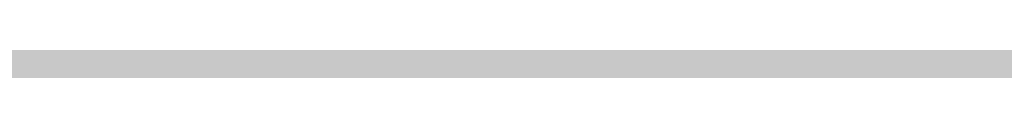
# Model space of a CAD drawing. Units: millimetres. Extents: x 0 to 2267, y 0 to 1823.
# Tile 242 of 256: x 1842.748 to 1843.095, y 1127.4185 to 1127.4234. Entities that reach past the tile are written whole.
import ezdxf

# ---------------------------------------------------------------- set-up
doc = ezdxf.new("R2010")
doc.units = ezdxf.units.MM
doc.header["$MEASUREMENT"] = 0
doc.layers.add('M-HATC', color=252, linetype='Continuous', lineweight=18)

msp = doc.modelspace()

# ---------------------------------------------------------------- hatches: boundary and pattern name
at = {"layer": 'M-HATC'}
h = msp.add_hatch(color=256, dxfattribs=at)
h.dxf.hatch_style = 1
h.paths.add_polyline_path([(2055.77105, 1603.06204), (1381.08677, 1603.06204), (1381.08677, 1598.06204), (2055.77105, 1598.06204)])
h.paths.add_polyline_path([(2055.77105, 1598.06204), (1381.08677, 1598.06204), (1381.08677, 1593.06204), (2055.77105, 1593.06204)])
h.paths.add_polyline_path([(2051.30737, 1536.76088), (1385.55044, 1536.76088), (1385.55044, 1526.76088), (1387.55044, 1526.76088), (1388.53662, 1525.05276), (1385.33187, 1521.23348), (1385.33187, 1521.22256), (2050.25417, 1522.74913), (2048.32119, 1525.05276), (2049.30737, 1526.76088), (2051.30737, 1526.76088)])
edge = h.paths.add_edge_path()
edge.add_arc((1847.53451, 1379.14917), 135, 222.6030607, 222.8908505, ccw=False)
edge.add_line((1748.16629, 1287.76561), (1683.09212, 1287.76561))
edge.add_arc((1583.7239, 1379.14917), 135, 317.1091495, 317.3969393, ccw=False)
edge.add_arc((1678.9686, 1290.67067), 5, 222.89085, 317.10915, ccw=False)
edge.add_arc((1774.21331, 1379.14917), 135, 222.6030607, 222.8908505, ccw=False)
edge.add_line((1674.84509, 1287.76561), (1609.77092, 1287.76561))
edge.add_arc((1510.4027, 1379.14917), 135, 317.1091495, 317.3969393, ccw=False)
edge.add_arc((1605.6474, 1290.67067), 5, 222.89085, 317.10915, ccw=False)
edge.add_arc((1700.89211, 1379.14917), 135, 222.6030607, 222.8908505, ccw=False)
edge.add_line((1601.52388, 1287.76561), (1536.44972, 1287.76561))
edge.add_arc((1437.08149, 1379.14917), 135, 317.1091495, 317.3969393, ccw=False)
edge.add_arc((1532.3262, 1290.67067), 5, 222.89085, 317.10915, ccw=False)
edge.add_arc((1627.57091, 1379.14917), 135, 222.6030607, 222.8908505, ccw=False)
edge.add_line((1528.20268, 1287.76561), (1505.92891, 1287.76561))
edge.add_spline(control_points=[(1505.92891, 1287.76561), (1504.26224, 1287.76561), (1504.26224, 1282.76561), (1505.92891, 1282.76561)], knot_values=[0, 0, 0, 0, 5, 5, 5, 5], degree=3, periodic=0)
edge.add_line((1505.92891, 1282.76561), (1930.92891, 1282.76561))
edge.add_spline(control_points=[(1930.92891, 1282.76561), (1932.59557, 1282.76561), (1932.59557, 1287.76561), (1930.92891, 1287.76561)], knot_values=[0, 0, 0, 0, 5, 5, 5, 5], degree=3, periodic=0)
edge.add_line((1930.92891, 1287.76561), (1903.05573, 1287.76561))
edge.add_arc((1803.6875, 1379.14917), 135, 317.1091495, 317.3969393, ccw=False)
edge.add_arc((1898.93221, 1290.67067), 5, 222.89085, 317.10915, ccw=False)
edge.add_arc((1994.17691, 1379.14917), 135, 222.6030607, 222.8908505, ccw=False)
edge.add_line((1894.80869, 1287.76561), (1829.73452, 1287.76561))
edge.add_arc((1730.3663, 1379.14917), 135, 317.1091495, 317.3969393, ccw=False)
edge.add_arc((1825.61101, 1290.67067), 5, 222.89085, 317.10915, ccw=False)
edge.add_arc((1920.85571, 1379.14917), 135, 222.6030607, 222.8908505, ccw=False)
edge.add_line((1821.48749, 1287.76561), (1756.41332, 1287.76561))
edge.add_arc((1657.0451, 1379.14917), 135, 317.1091495, 317.3969393, ccw=False)
edge.add_arc((1752.28981, 1290.67067), 5, 222.89085, 317.10915, ccw=False)
edge = h.paths.add_edge_path()
edge.add_spline(control_points=[(1843.42891, 1227.24746), (1845.09557, 1227.24746), (1845.09557, 1232.24746), (1843.42891, 1232.24746)], knot_values=[0, 0, 0, 0, 5, 5, 5, 5], degree=3, periodic=0)
edge.add_line((1843.42891, 1232.24746), (1593.42891, 1232.24746))
edge.add_spline(control_points=[(1593.42891, 1232.24746), (1591.76224, 1232.24746), (1591.76224, 1227.24746), (1593.42891, 1227.24746)], knot_values=[0, 0, 0, 0, 5, 5, 5, 5], degree=3, periodic=0)
edge.add_line((1593.42891, 1227.24746), (1843.42891, 1227.24746))
h.paths.add_polyline_path([(1905.92891, 1127.41706), (1530.92891, 1127.41706, 0.414214), (1520.92891, 1117.41706), (1530.92891, 1117.41706), (1915.92891, 1117.41706, 0.414214)])
edge = h.paths.add_edge_path()
edge.add_arc((1397.08577, 1498.40775), 12.72993, 90.782146, 190.878706, ccw=False)
edge.add_line((1396.912, 1511.13649), (1428.00968, 1511.34875))
edge.add_line((1428.00968, 1511.34875), (1433.00968, 1511.34875))
edge.add_line((1433.00968, 1511.34875), (1434.439, 1511.34875))
edge.add_arc((1419.474, 1498.08041), 20, 41.560995, 74.082109)
edge.add_line((1424.95919, 1517.31353), (1399.93509, 1517.25608))
edge.add_spline(control_points=[(1399.93074, 1517.25607), (1399.88398, 1517.21312), (1399.8328, 1517.16893), (1399.77741, 1517.1236)], knot_values=[11.567499, 11.567499, 11.567499, 11.567499, 11.814249, 11.814249, 11.814249, 11.814249], degree=3, periodic=0)
edge.add_spline(control_points=[(1399.63279, 1517.00986), (1399.58305, 1516.97214), (1399.53072, 1516.93375), (1399.47591, 1516.89474)], knot_values=[11.167718, 11.167718, 11.167718, 11.167718, 11.365188, 11.365188, 11.365188, 11.365188], degree=3, periodic=0)
edge.add_spline(control_points=[(1399.33981, 1516.80007), (1399.15144, 1516.67185), (1398.93836, 1516.5377), (1398.70404, 1516.39942)], knot_values=[10.376405, 10.376405, 10.376405, 10.376405, 11.00994, 11.00994, 11.00994, 11.00994], degree=3, periodic=0)
edge.add_spline(control_points=[(1398.65716, 1516.37187), (1398.57885, 1516.32602), (1398.49825, 1516.27974), (1398.41549, 1516.23309)], knot_values=[10.125175, 10.125175, 10.125175, 10.125175, 10.334406, 10.334406, 10.334406, 10.334406], degree=3, periodic=0)
edge.add_spline(control_points=[(1398.26422, 1516.14874), (1398.19595, 1516.11107), (1398.12634, 1516.07319), (1398.05546, 1516.03513)], knot_values=[9.832246, 9.832246, 9.832246, 9.832246, 9.999658, 9.999658, 9.999658, 9.999658], degree=3, periodic=0)
edge.add_spline(control_points=[(1397.9987, 1516.00476), (1397.73115, 1515.86211), (1397.44602, 1515.71707), (1397.14664, 1515.57138)], knot_values=[9.161808, 9.161808, 9.161808, 9.161808, 9.787769, 9.787769, 9.787769, 9.787769], degree=3, periodic=0)
edge.add_spline(control_points=[(1397.14664, 1515.57138), (1396.84182, 1515.42305), (1396.52223, 1515.27404), (1396.1914, 1515.12621)], knot_values=[8.524455, 8.524455, 8.524455, 8.524455, 9.161808, 9.161808, 9.161808, 9.161808], degree=3, periodic=0)
edge.add_spline(control_points=[(1396.07771, 1515.07565), (1395.98538, 1515.03478), (1395.89222, 1514.99402), (1395.7983, 1514.9534)], knot_values=[8.275193, 8.275193, 8.275193, 8.275193, 8.451726, 8.451726, 8.451726, 8.451726], degree=3, periodic=0)
edge.add_spline(control_points=[(1395.60184, 1514.86912), (1395.49975, 1514.82568), (1395.39685, 1514.78244), (1395.29322, 1514.73944)], knot_values=[7.962917, 7.962917, 7.962917, 7.962917, 8.152764, 8.152764, 8.152764, 8.152764], degree=3, periodic=0)
edge.add_spline(control_points=[(1395.21158, 1514.70568), (1394.82779, 1514.5475), (1394.43452, 1514.39287), (1394.03645, 1514.24422)], knot_values=[7.21254, 7.21254, 7.21254, 7.21254, 7.913148, 7.913148, 7.913148, 7.913148], degree=3, periodic=0)
edge.add_spline(control_points=[(1394.03645, 1514.24422), (1393.70758, 1514.12142), (1393.37544, 1514.0027), (1393.04267, 1513.88945)], knot_values=[6.633733, 6.633733, 6.633733, 6.633733, 7.21254, 7.21254, 7.21254, 7.21254], degree=3, periodic=0)
edge.add_spline(control_points=[(1392.82142, 1513.81499), (1392.71978, 1513.78118), (1392.61815, 1513.74791), (1392.51658, 1513.71521)], knot_values=[6.328796, 6.328796, 6.328796, 6.328796, 6.505493, 6.505493, 6.505493, 6.505493], degree=3, periodic=0)
edge.add_spline(control_points=[(1392.51658, 1513.71521), (1392.31873, 1513.65151), (1392.12116, 1513.59001), (1391.92441, 1513.53098)], knot_values=[5.984605, 5.984605, 5.984605, 5.984605, 6.328796, 6.328796, 6.328796, 6.328796], degree=3, periodic=0)
edge.add_spline(control_points=[(1391.79155, 1513.49146), (1391.31215, 1513.35011), (1390.83842, 1513.22392), (1390.37844, 1513.11711)], knot_values=[5.066697, 5.066697, 5.066697, 5.066697, 5.907055, 5.907055, 5.907055, 5.907055], degree=3, periodic=0)
edge.add_spline(control_points=[(1390.37844, 1513.11711), (1390.17973, 1513.07097), (1389.98359, 1513.02845), (1389.79067, 1512.98988)], knot_values=[4.70367, 4.70367, 4.70367, 4.70367, 5.066695, 5.066695, 5.066695, 5.066695], degree=3, periodic=0)
edge.add_spline(control_points=[(1389.42203, 1512.92036), (1389.24588, 1512.88922), (1389.0729, 1512.86172), (1388.90364, 1512.83814)], knot_values=[4.130571, 4.130571, 4.130571, 4.130571, 4.469816, 4.469816, 4.469816, 4.469816], degree=3, periodic=0)
edge.add_spline(control_points=[(1388.90364, 1512.83814), (1388.59103, 1512.7946), (1388.29108, 1512.76444), (1388.00714, 1512.74941)], knot_values=[3.504031, 3.504031, 3.504031, 3.504031, 4.130571, 4.130571, 4.130571, 4.130571], degree=3, periodic=0)
edge.add_spline(control_points=[(1387.9356, 1512.74593), (1387.85378, 1512.74231), (1387.77334, 1512.73997), (1387.69435, 1512.73898)], knot_values=[3.268866, 3.268866, 3.268866, 3.268866, 3.451164, 3.451164, 3.451164, 3.451164], degree=3, periodic=0)
edge.add_spline(control_points=[(1387.33512, 1512.74426), (1387.20757, 1512.74991), (1387.08472, 1512.7597), (1386.96699, 1512.77385)], knot_values=[2.670686, 2.670686, 2.670686, 2.670686, 2.984, 2.984, 2.984, 2.984], degree=3, periodic=0)
edge.add_spline(control_points=[(1386.83274, 1512.79225), (1386.82093, 1512.79407), (1386.80917, 1512.79594), (1386.79747, 1512.79787)], knot_values=[2.516981, 2.516981, 2.516981, 2.516981, 2.549528, 2.549528, 2.549528, 2.549528], degree=3, periodic=0)
edge.add_spline(control_points=[(1386.45257, 1512.87348), (1386.42573, 1512.88105), (1386.39931, 1512.88895), (1386.3733, 1512.89719)], knot_values=[2.095869, 2.095869, 2.095869, 2.095869, 2.17941, 2.17941, 2.17941, 2.17941], degree=3, periodic=0)
edge.add_spline(control_points=[(1386.06911, 1513.01889), (1386.06338, 1513.02174), (1386.05768, 1513.02463), (1386.05201, 1513.02753)], knot_values=[1.72453, 1.72453, 1.72453, 1.72453, 1.745933, 1.745933, 1.745933, 1.745933], degree=3, periodic=0)
edge.add_arc((1399.474, 1498.08041), 20, 131.824322, 180)
edge.add_arc((1630.33362, 1505.54843), 250.97076, 181.7051759, 236.427975)
edge.add_arc((1605.33992, 1483.30441), 218.7822, 238.660829, 243.3496099)
edge.add_arc((1647.09105, 1510.35917), 262.89859, 183.1298361, 237.8534422, ccw=False)
h.paths.add_polyline_path([(1406.53685, 1391.96444, 0.149382), (1491.55061, 1296.44177, -0.129517)], flags=17)
edge = h.paths.add_edge_path()
edge.add_arc((2037.38381, 1498.08041), 20, 0, 48.265868)
edge.add_spline(control_points=[(2050.69731, 1513.00525), (2050.65121, 1512.98471), (2050.60338, 1512.96554), (2050.55388, 1512.94771)], knot_values=[1.835652, 1.835652, 1.835652, 1.835652, 2.000781, 2.000781, 2.000781, 2.000781], degree=3, periodic=0)
edge.add_spline(control_points=[(2050.46156, 1512.91661), (2050.479, 1512.9221), (2050.49625, 1512.92774), (2050.51332, 1512.93353)], knot_values=[2.045477, 2.045477, 2.045477, 2.045477, 2.101389, 2.101389, 2.101389, 2.101389], degree=3, periodic=0)
edge.add_spline(control_points=[(2050.12896, 1512.83416), (2050.19843, 1512.84734), (2050.26573, 1512.86233), (2050.33075, 1512.87919)], knot_values=[2.237629, 2.237629, 2.237629, 2.237629, 2.435841, 2.435841, 2.435841, 2.435841], degree=3, periodic=0)
edge.add_spline(control_points=[(2050.09463, 1512.82783), (2050.10613, 1512.82989), (2050.11757, 1512.832), (2050.12896, 1512.83416)], knot_values=[2.435841, 2.435841, 2.435841, 2.435841, 2.468321, 2.468321, 2.468321, 2.468321], degree=3, periodic=0)
edge.add_spline(control_points=[(2049.78433, 1512.78511), (2049.85521, 1512.79219), (2049.92435, 1512.80077), (2049.99166, 1512.81088)], knot_values=[2.563852, 2.563852, 2.563852, 2.563852, 2.748541, 2.748541, 2.748541, 2.748541], degree=3, periodic=0)
edge.add_spline(control_points=[(2049.4052, 1512.76169), (2049.5364, 1512.76526), (2049.66292, 1512.77299), (2049.78433, 1512.78511)], knot_values=[2.748541, 2.748541, 2.748541, 2.748541, 3.064882, 3.064882, 3.064882, 3.064882], degree=3, periodic=0)
edge.add_spline(control_points=[(2049.16976, 1512.75968), (2049.23364, 1512.7591), (2049.29654, 1512.7594), (2049.35844, 1512.7606)], knot_values=[3.102309, 3.102309, 3.102309, 3.102309, 3.2503, 3.2503, 3.2503, 3.2503], degree=3, periodic=0)
edge.add_spline(control_points=[(2048.85727, 1512.76911), (2048.96378, 1512.76378), (2049.068, 1512.76061), (2049.16976, 1512.75968)], knot_values=[3.2503, 3.2503, 3.2503, 3.2503, 3.486069, 3.486069, 3.486069, 3.486069], degree=3, periodic=0)
edge.add_spline(control_points=[(2048.69241, 1512.77892), (2048.3729, 1512.80093), (2048.0345, 1512.84106), (2047.68175, 1512.89697)], knot_values=[3.606429, 3.606429, 3.606429, 3.606429, 4.2989, 4.2989, 4.2989, 4.2989], degree=3, periodic=0)
edge.add_spline(control_points=[(2047.68175, 1512.89697), (2047.5458, 1512.91852), (2047.40772, 1512.94241), (2047.26776, 1512.96851)], knot_values=[4.2989, 4.2989, 4.2989, 4.2989, 4.565769, 4.565769, 4.565769, 4.565769], degree=3, periodic=0)
edge.add_spline(control_points=[(2047.26776, 1512.96851), (2047.14494, 1512.99141), (2047.02067, 1513.01601), (2046.89514, 1513.04223)], knot_values=[4.565769, 4.565769, 4.565769, 4.565769, 4.799971, 4.799971, 4.799971, 4.799971], degree=3, periodic=0)
edge.add_spline(control_points=[(2046.89514, 1513.04223), (2046.52865, 1513.11875), (2046.15135, 1513.20899), (2045.7676, 1513.31068)], knot_values=[4.799971, 4.799971, 4.799971, 4.799971, 5.483718, 5.483718, 5.483718, 5.483718], degree=3, periodic=0)
edge.add_spline(control_points=[(2045.7676, 1513.31068), (2045.3724, 1513.41539), (2044.97036, 1513.53225), (2044.56625, 1513.65876)], knot_values=[5.483718, 5.483718, 5.483718, 5.483718, 6.187866, 6.187866, 6.187866, 6.187866], degree=3, periodic=0)
edge.add_spline(control_points=[(2044.56625, 1513.65876), (2044.41491, 1513.70614), (2044.26329, 1513.75487), (2044.11163, 1513.80482)], knot_values=[6.187866, 6.187866, 6.187866, 6.187866, 6.451551, 6.451551, 6.451551, 6.451551], degree=3, periodic=0)
edge.add_spline(control_points=[(2044.11163, 1513.80482), (2043.99666, 1513.84269), (2043.88167, 1513.88126), (2043.76676, 1513.92048)], knot_values=[6.451551, 6.451551, 6.451551, 6.451551, 6.651434, 6.651434, 6.651434, 6.651434], degree=3, periodic=0)
edge.add_spline(control_points=[(2043.76676, 1513.92048), (2043.37157, 1514.05536), (2042.97738, 1514.19789), (2042.58863, 1514.34575)], knot_values=[6.651434, 6.651434, 6.651434, 6.651434, 7.338879, 7.338879, 7.338879, 7.338879], degree=3, periodic=0)
edge.add_spline(control_points=[(2042.58863, 1514.34575), (2042.16431, 1514.50715), (2041.74647, 1514.67491), (2041.34086, 1514.84603)], knot_values=[7.338879, 7.338879, 7.338879, 7.338879, 8.089209, 8.089209, 8.089209, 8.089209], degree=3, periodic=0)
edge.add_spline(control_points=[(2041.34086, 1514.84603), (2041.1028, 1514.94647), (2040.86896, 1515.04806), (2040.64049, 1515.1502)], knot_values=[8.089209, 8.089209, 8.089209, 8.089209, 8.529587, 8.529587, 8.529587, 8.529587], degree=3, periodic=0)
edge.add_spline(control_points=[(2040.50999, 1515.20887), (2040.08238, 1515.40218), (2039.67475, 1515.59705), (2039.29495, 1515.78939)], knot_values=[8.613818, 8.613818, 8.613818, 8.613818, 9.44571, 9.44571, 9.44571, 9.44571], degree=3, periodic=0)
edge.add_spline(control_points=[(2039.29495, 1515.78939), (2039.0618, 1515.90746), (2038.83914, 1516.02458), (2038.62878, 1516.1398)], knot_values=[9.44571, 9.44571, 9.44571, 9.44571, 9.956404, 9.956404, 9.956404, 9.956404], degree=3, periodic=0)
edge.add_spline(control_points=[(2038.62878, 1516.1398), (2038.51874, 1516.20007), (2038.41207, 1516.25982), (2038.30903, 1516.31891)], knot_values=[9.956404, 9.956404, 9.956404, 9.956404, 10.223542, 10.223542, 10.223542, 10.223542], degree=3, periodic=0)
edge.add_spline(control_points=[(2038.30903, 1516.31891), (2038.21377, 1516.37354), (2038.12161, 1516.42762), (2038.03275, 1516.48102)], knot_values=[10.223542, 10.223542, 10.223542, 10.223542, 10.47051, 10.47051, 10.47051, 10.47051], degree=3, periodic=0)
edge.add_spline(control_points=[(2038.03275, 1516.48102), (2037.78552, 1516.62961), (2037.56388, 1516.77304), (2037.37225, 1516.909)], knot_values=[10.47051, 10.47051, 10.47051, 10.47051, 11.15767, 11.15767, 11.15767, 11.15767], degree=3, periodic=0)
edge.add_spline(control_points=[(2037.37225, 1516.909), (2037.27893, 1516.9752), (2037.19274, 1517.03963), (2037.11417, 1517.10203)], knot_values=[11.15767, 11.15767, 11.15767, 11.15767, 11.49227, 11.49227, 11.49227, 11.49227], degree=3, periodic=0)
edge.add_spline(control_points=[(2036.85638, 1517.32585), (2036.91481, 1517.26923), (2036.98143, 1517.21027), (2037.05573, 1517.14922)], knot_values=[11.577341, 11.577341, 11.577341, 11.577341, 11.91035, 11.91035, 11.91035, 11.91035], degree=3, periodic=0)
edge.add_spline(control_points=[(2036.80739, 1517.37475), (2036.82301, 1517.35865), (2036.83935, 1517.34235), (2036.85638, 1517.32585)], knot_values=[11.91035, 11.91035, 11.91035, 11.91035, 12.007402, 12.007402, 12.007402, 12.007402], degree=3, periodic=0)
edge.add_spline(control_points=[(2036.70167, 1517.494), (2036.71042, 1517.48299), (2036.71958, 1517.47185), (2036.72913, 1517.4606)], knot_values=[12.184155, 12.184155, 12.184155, 12.184155, 12.255409, 12.255409, 12.255409, 12.255409], degree=3, periodic=0)
edge.add_spline(control_points=[(2036.6159, 1517.6205), (2036.61998, 1517.61304), (2036.6243, 1517.6055), (2036.62885, 1517.59789)], knot_values=[12.487913, 12.487913, 12.487913, 12.487913, 12.541035, 12.541035, 12.541035, 12.541035], degree=3, periodic=0)
edge.add_spline(control_points=[(2036.56349, 1517.78599), (2036.56372, 1517.77936), (2036.56423, 1517.77264), (2036.56502, 1517.76582)], knot_values=[12.911761, 12.911761, 12.911761, 12.911761, 12.968286, 12.968286, 12.968286, 12.968286], degree=3, periodic=0)
edge.add_spline(control_points=[(2036.61663, 1517.93042), (2036.61248, 1517.92586), (2036.60857, 1517.92121), (2036.60491, 1517.91648)], knot_values=[13.382527, 13.382527, 13.382527, 13.382527, 13.433791, 13.433791, 13.433791, 13.433791], degree=3, periodic=0)
edge.add_spline(control_points=[(2036.74902, 1518.01695), (2036.73613, 1518.0116), (2036.72393, 1518.00601), (2036.71242, 1518.00018)], knot_values=[13.726299, 13.726299, 13.726299, 13.726299, 13.809928, 13.809928, 13.809928, 13.809928], degree=3, periodic=0)
edge.add_spline(control_points=[(2036.86043, 1518.05285), (2036.83863, 1518.04743), (2036.81809, 1518.04156), (2036.79879, 1518.03526)], knot_values=[13.910887, 13.910887, 13.910887, 13.910887, 14.02153, 14.02153, 14.02153, 14.02153], degree=3, periodic=0)
edge.add_line((2036.96387, 1518.08041), (2032.38381, 1518.08041))
edge.add_line((2032.38381, 1518.08041), (2027.38381, 1518.08041))
edge.add_line((2027.38381, 1518.08041), (2022.38381, 1518.08041))
edge.add_line((2022.38381, 1518.08041), (2017.38381, 1518.08041))
edge.add_arc((2017.38381, 1498.08041), 20, 90, 138.439005)
edge.add_line((2002.41881, 1511.34875), (2003.84813, 1511.34875))
edge.add_line((2003.84813, 1511.34875), (2008.84813, 1511.34875))
edge.add_line((2008.84813, 1511.34875), (2039.77204, 1511.13768))
edge.add_arc((2039.77204, 1498.40775), 12.72993, -10.878706, 90, ccw=False)
edge.add_arc((1789.76676, 1510.35917), 262.89859, 302.1465578, 356.8701639, ccw=False)
edge.add_arc((1831.51789, 1483.30441), 218.7822, 296.6503901, 301.339171)
edge.add_arc((1806.52419, 1505.54843), 250.97076, 303.572025, 358.2948241)
h.paths.add_polyline_path([(2030.32096, 1391.96444, -0.129517), (1945.3072, 1296.44177, 0.149382)], flags=17)
edge = h.paths.add_edge_path()
edge.add_spline(control_points=[(2037.2464, 1518.08209), (2037.28977, 1518.08098), (2037.33555, 1518.08041), (2037.3838, 1518.08041)], knot_values=[0.000012, 0.000012, 0.000012, 0.000012, 0.144754, 0.144754, 0.144754, 0.144754], degree=3, periodic=0)
edge.add_line((2037.33571, 1518.08041), (2037.00963, 1518.08041))
edge.add_spline(control_points=[(2037.00963, 1518.08041), (2036.98217, 1518.07678), (2036.95605, 1518.07266), (2036.93124, 1518.06808)], knot_values=[14.13465, 14.13465, 14.13465, 14.13465, 14.247197, 14.247197, 14.247197, 14.247197], degree=3, periodic=0)
edge.add_spline(control_points=[(2036.93124, 1518.06808), (2036.92764, 1518.06741), (2036.92407, 1518.06674), (2036.92053, 1518.06605)], knot_values=[14.118315, 14.118315, 14.118315, 14.118315, 14.13465, 14.13465, 14.13465, 14.13465], degree=3, periodic=0)
edge.add_spline(control_points=[(2036.92053, 1518.06605), (2036.9118, 1518.06436), (2036.90323, 1518.06262), (2036.89484, 1518.06081)], knot_values=[14.078086, 14.078086, 14.078086, 14.078086, 14.118315, 14.118315, 14.118315, 14.118315], degree=3, periodic=0)
edge.add_spline(control_points=[(2036.89484, 1518.06081), (2036.88304, 1518.05827), (2036.87157, 1518.05562), (2036.86043, 1518.05285)], knot_values=[14.02153, 14.02153, 14.02153, 14.02153, 14.078086, 14.078086, 14.078086, 14.078086], degree=3, periodic=0)
edge.add_spline(control_points=[(2036.86043, 1518.05285), (2036.83863, 1518.04743), (2036.81809, 1518.04156), (2036.79879, 1518.03526)], knot_values=[13.910887, 13.910887, 13.910887, 13.910887, 14.02153, 14.02153, 14.02153, 14.02153], degree=3, periodic=0)
edge.add_spline(control_points=[(2036.79879, 1518.03526), (2036.79809, 1518.03504), (2036.7974, 1518.03481), (2036.79671, 1518.03458)], knot_values=[13.906906, 13.906906, 13.906906, 13.906906, 13.910887, 13.910887, 13.910887, 13.910887], degree=3, periodic=0)
edge.add_spline(control_points=[(2036.79671, 1518.03458), (2036.78819, 1518.03178), (2036.77991, 1518.02888), (2036.77187, 1518.02591)], knot_values=[13.857826, 13.857826, 13.857826, 13.857826, 13.906906, 13.906906, 13.906906, 13.906906], degree=3, periodic=0)
edge.add_spline(control_points=[(2036.77187, 1518.02591), (2036.76402, 1518.023), (2036.75641, 1518.02002), (2036.74902, 1518.01695)], knot_values=[13.809928, 13.809928, 13.809928, 13.809928, 13.857826, 13.857826, 13.857826, 13.857826], degree=3, periodic=0)
edge.add_spline(control_points=[(2036.74902, 1518.01695), (2036.73613, 1518.0116), (2036.72393, 1518.00601), (2036.71242, 1518.00018)], knot_values=[13.726299, 13.726299, 13.726299, 13.726299, 13.809928, 13.809928, 13.809928, 13.809928], degree=3, periodic=0)
edge.add_spline(control_points=[(2036.71242, 1518.00018), (2036.71211, 1518.00002), (2036.71179, 1517.99986), (2036.71147, 1517.99969)], knot_values=[13.723993, 13.723993, 13.723993, 13.723993, 13.726299, 13.726299, 13.726299, 13.726299], degree=3, periodic=0)
edge.add_spline(control_points=[(2036.71147, 1517.99969), (2036.70634, 1517.99708), (2036.70134, 1517.99441), (2036.69648, 1517.9917)], knot_values=[13.686536, 13.686536, 13.686536, 13.686536, 13.723993, 13.723993, 13.723993, 13.723993], degree=3, periodic=0)
edge.add_spline(control_points=[(2036.69648, 1517.9917), (2036.6919, 1517.98914), (2036.68744, 1517.98654), (2036.6831, 1517.9839)], knot_values=[13.651251, 13.651251, 13.651251, 13.651251, 13.686536, 13.686536, 13.686536, 13.686536], degree=3, periodic=0)
edge.add_spline(control_points=[(2036.6831, 1517.9839), (2036.67641, 1517.97983), (2036.67001, 1517.97566), (2036.6639, 1517.97139)], knot_values=[13.596804, 13.596804, 13.596804, 13.596804, 13.651251, 13.651251, 13.651251, 13.651251], degree=3, periodic=0)
edge.add_spline(control_points=[(2036.6639, 1517.97139), (2036.66358, 1517.97117), (2036.66326, 1517.97094), (2036.66294, 1517.97072)], knot_values=[13.593956, 13.593956, 13.593956, 13.593956, 13.596804, 13.596804, 13.596804, 13.596804], degree=3, periodic=0)
edge.add_spline(control_points=[(2036.66294, 1517.97072), (2036.6603, 1517.96886), (2036.65771, 1517.96698), (2036.65518, 1517.96509)], knot_values=[13.570322, 13.570322, 13.570322, 13.570322, 13.593956, 13.593956, 13.593956, 13.593956], degree=3, periodic=0)
edge.add_spline(control_points=[(2036.65518, 1517.96509), (2036.65251, 1517.9631), (2036.64991, 1517.96108), (2036.64737, 1517.95905)], knot_values=[13.545477, 13.545477, 13.545477, 13.545477, 13.570322, 13.570322, 13.570322, 13.570322], degree=3, periodic=0)
edge.add_spline(control_points=[(2036.64737, 1517.95905), (2036.64721, 1517.95892), (2036.64705, 1517.9588), (2036.64689, 1517.95867)], knot_values=[13.543931, 13.543931, 13.543931, 13.543931, 13.545477, 13.545477, 13.545477, 13.545477], degree=3, periodic=0)
edge.add_spline(control_points=[(2036.64689, 1517.95867), (2036.64121, 1517.95411), (2036.63582, 1517.94945), (2036.63073, 1517.94468)], knot_values=[13.488237, 13.488237, 13.488237, 13.488237, 13.543931, 13.543931, 13.543931, 13.543931], degree=3, periodic=0)
edge.add_spline(control_points=[(2036.63073, 1517.94468), (2036.62817, 1517.94229), (2036.62569, 1517.93988), (2036.62329, 1517.93744)], knot_values=[13.460307, 13.460307, 13.460307, 13.460307, 13.488237, 13.488237, 13.488237, 13.488237], degree=3, periodic=0)
edge.add_spline(control_points=[(2036.62329, 1517.93744), (2036.62151, 1517.93564), (2036.61978, 1517.93383), (2036.61809, 1517.932)], knot_values=[13.439712, 13.439712, 13.439712, 13.439712, 13.460307, 13.460307, 13.460307, 13.460307], degree=3, periodic=0)
edge.add_spline(control_points=[(2036.61809, 1517.932), (2036.6176, 1517.93147), (2036.61711, 1517.93095), (2036.61663, 1517.93042)], knot_values=[13.433791, 13.433791, 13.433791, 13.433791, 13.439712, 13.439712, 13.439712, 13.439712], degree=3, periodic=0)
edge.add_spline(control_points=[(2036.61663, 1517.93042), (2036.61248, 1517.92586), (2036.60857, 1517.92121), (2036.60491, 1517.91648)], knot_values=[13.382527, 13.382527, 13.382527, 13.382527, 13.433791, 13.433791, 13.433791, 13.433791], degree=3, periodic=0)
edge.add_spline(control_points=[(2036.60491, 1517.91648), (2036.60258, 1517.91347), (2036.60036, 1517.91044), (2036.59824, 1517.90737)], knot_values=[13.350017, 13.350017, 13.350017, 13.350017, 13.382527, 13.382527, 13.382527, 13.382527], degree=3, periodic=0)
edge.add_spline(control_points=[(2036.59824, 1517.90737), (2036.59718, 1517.90585), (2036.59616, 1517.90433), (2036.59515, 1517.90279)], knot_values=[13.333922, 13.333922, 13.333922, 13.333922, 13.350017, 13.350017, 13.350017, 13.350017], degree=3, periodic=0)
edge.add_spline(control_points=[(2036.59515, 1517.90279), (2036.59452, 1517.90183), (2036.5939, 1517.90086), (2036.59329, 1517.89989)], knot_values=[13.323828, 13.323828, 13.323828, 13.323828, 13.333922, 13.333922, 13.333922, 13.333922], degree=3, periodic=0)
edge.add_spline(control_points=[(2036.59329, 1517.89989), (2036.59049, 1517.89545), (2036.5879, 1517.89094), (2036.5855, 1517.88637)], knot_values=[13.277545, 13.277545, 13.277545, 13.277545, 13.323828, 13.323828, 13.323828, 13.323828], degree=3, periodic=0)
edge.add_spline(control_points=[(2036.5855, 1517.88637), (2036.58355, 1517.88267), (2036.58174, 1517.87892), (2036.58006, 1517.87513)], knot_values=[13.240119, 13.240119, 13.240119, 13.240119, 13.277545, 13.277545, 13.277545, 13.277545], degree=3, periodic=0)
edge.add_spline(control_points=[(2036.58006, 1517.87513), (2036.57952, 1517.87393), (2036.579, 1517.87272), (2036.57849, 1517.87151)], knot_values=[13.228211, 13.228211, 13.228211, 13.228211, 13.240119, 13.240119, 13.240119, 13.240119], degree=3, periodic=0)
edge.add_spline(control_points=[(2036.57849, 1517.87151), (2036.57796, 1517.87023), (2036.57744, 1517.86896), (2036.57693, 1517.86767)], knot_values=[13.215717, 13.215717, 13.215717, 13.215717, 13.228211, 13.228211, 13.228211, 13.228211], degree=3, periodic=0)
edge.add_spline(control_points=[(2036.57693, 1517.86767), (2036.57548, 1517.86399), (2036.57414, 1517.86027), (2036.57293, 1517.85651)], knot_values=[13.179847, 13.179847, 13.179847, 13.179847, 13.215717, 13.215717, 13.215717, 13.215717], degree=3, periodic=0)
edge.add_spline(control_points=[(2036.57293, 1517.85651), (2036.5713, 1517.8515), (2036.56989, 1517.84641), (2036.56868, 1517.84126)], knot_values=[13.132017, 13.132017, 13.132017, 13.132017, 13.179847, 13.179847, 13.179847, 13.179847], degree=3, periodic=0)
edge.add_spline(control_points=[(2036.56868, 1517.84126), (2036.56844, 1517.84023), (2036.56821, 1517.8392), (2036.56798, 1517.83817)], knot_values=[13.122482, 13.122482, 13.122482, 13.122482, 13.132017, 13.132017, 13.132017, 13.132017], degree=3, periodic=0)
edge.add_spline(control_points=[(2036.56798, 1517.83817), (2036.56758, 1517.83634), (2036.56721, 1517.8345), (2036.56687, 1517.83266)], knot_values=[13.105592, 13.105592, 13.105592, 13.105592, 13.122482, 13.122482, 13.122482, 13.122482], degree=3, periodic=0)
edge.add_spline(control_points=[(2036.56687, 1517.83266), (2036.56622, 1517.82921), (2036.56567, 1517.82574), (2036.5652, 1517.82223)], knot_values=[13.074063, 13.074063, 13.074063, 13.074063, 13.105592, 13.105592, 13.105592, 13.105592], degree=3, periodic=0)
edge.add_spline(control_points=[(2036.5652, 1517.82223), (2036.5652, 1517.82223), (2036.5652, 1517.82223), (2036.5652, 1517.82223)], knot_values=[13.074043, 13.074043, 13.074043, 13.074043, 13.074063, 13.074063, 13.074063, 13.074063], degree=3, periodic=0)
edge.add_spline(control_points=[(2036.5652, 1517.82223), (2036.56443, 1517.81643), (2036.5639, 1517.81055), (2036.56361, 1517.8046)], knot_values=[13.021884, 13.021884, 13.021884, 13.021884, 13.074043, 13.074043, 13.074043, 13.074043], degree=3, periodic=0)
edge.add_spline(control_points=[(2036.56361, 1517.8046), (2036.56358, 1517.80401), (2036.56356, 1517.80342), (2036.56353, 1517.80283)], knot_values=[13.01674, 13.01674, 13.01674, 13.01674, 13.021884, 13.021884, 13.021884, 13.021884], degree=3, periodic=0)
edge.add_spline(control_points=[(2036.56353, 1517.80283), (2036.56344, 1517.80051), (2036.56338, 1517.79817), (2036.56336, 1517.79582)], knot_values=[12.996438, 12.996438, 12.996438, 12.996438, 13.01674, 13.01674, 13.01674, 13.01674], degree=3, periodic=0)
edge.add_spline(control_points=[(2036.56336, 1517.79582), (2036.56334, 1517.79257), (2036.56338, 1517.78929), (2036.56349, 1517.78599)], knot_values=[12.968286, 12.968286, 12.968286, 12.968286, 12.996438, 12.996438, 12.996438, 12.996438], degree=3, periodic=0)
edge.add_spline(control_points=[(2036.56349, 1517.78599), (2036.56372, 1517.77936), (2036.56423, 1517.77264), (2036.56502, 1517.76582)], knot_values=[12.911761, 12.911761, 12.911761, 12.911761, 12.968286, 12.968286, 12.968286, 12.968286], degree=3, periodic=0)
edge.add_spline(control_points=[(2036.56502, 1517.76582), (2036.56503, 1517.76573), (2036.56504, 1517.76564), (2036.56505, 1517.76555)], knot_values=[12.911017, 12.911017, 12.911017, 12.911017, 12.911761, 12.911761, 12.911761, 12.911761], degree=3, periodic=0)
edge.add_spline(control_points=[(2036.56505, 1517.76555), (2036.56541, 1517.76245), (2036.56583, 1517.75933), (2036.56631, 1517.75619)], knot_values=[12.88528, 12.88528, 12.88528, 12.88528, 12.911017, 12.911017, 12.911017, 12.911017], degree=3, periodic=0)
edge.add_spline(control_points=[(2036.56631, 1517.75619), (2036.56673, 1517.75341), (2036.5672, 1517.75062), (2036.56771, 1517.74782)], knot_values=[12.862519, 12.862519, 12.862519, 12.862519, 12.88528, 12.88528, 12.88528, 12.88528], degree=3, periodic=0)
edge.add_spline(control_points=[(2036.56771, 1517.74782), (2036.56779, 1517.74737), (2036.56788, 1517.74692), (2036.56796, 1517.74647)], knot_values=[12.858885, 12.858885, 12.858885, 12.858885, 12.862519, 12.862519, 12.862519, 12.862519], degree=3, periodic=0)
edge.add_spline(control_points=[(2036.56796, 1517.74647), (2036.5692, 1517.73986), (2036.57069, 1517.73316), (2036.57243, 1517.72638)], knot_values=[12.8053, 12.8053, 12.8053, 12.8053, 12.858885, 12.858885, 12.858885, 12.858885], degree=3, periodic=0)
edge.add_spline(control_points=[(2036.57243, 1517.72638), (2036.5734, 1517.72257), (2036.57446, 1517.71874), (2036.57559, 1517.71488)], knot_values=[12.775176, 12.775176, 12.775176, 12.775176, 12.8053, 12.8053, 12.8053, 12.8053], degree=3, periodic=0)
edge.add_spline(control_points=[(2036.57559, 1517.71488), (2036.57628, 1517.71252), (2036.577, 1517.71015), (2036.57775, 1517.70778)], knot_values=[12.756759, 12.756759, 12.756759, 12.756759, 12.775176, 12.775176, 12.775176, 12.775176], degree=3, periodic=0)
edge.add_spline(control_points=[(2036.57775, 1517.70778), (2036.57808, 1517.70674), (2036.57841, 1517.7057), (2036.57875, 1517.70466)], knot_values=[12.748742, 12.748742, 12.748742, 12.748742, 12.756759, 12.756759, 12.756759, 12.756759], degree=3, periodic=0)
edge.add_spline(control_points=[(2036.57875, 1517.70466), (2036.58082, 1517.6983), (2036.58309, 1517.69187), (2036.58557, 1517.68537)], knot_values=[12.69959, 12.69959, 12.69959, 12.69959, 12.748742, 12.748742, 12.748742, 12.748742], degree=3, periodic=0)
edge.add_spline(control_points=[(2036.58557, 1517.68537), (2036.58762, 1517.68001), (2036.5898, 1517.6746), (2036.59213, 1517.66916)], knot_values=[12.659038, 12.659038, 12.659038, 12.659038, 12.69959, 12.69959, 12.69959, 12.69959], degree=3, periodic=0)
edge.add_spline(control_points=[(2036.59213, 1517.66916), (2036.59397, 1517.66482), (2036.59591, 1517.66047), (2036.59793, 1517.65608)], knot_values=[12.626806, 12.626806, 12.626806, 12.626806, 12.659038, 12.659038, 12.659038, 12.659038], degree=3, periodic=0)
edge.add_spline(control_points=[(2036.59793, 1517.65608), (2036.59839, 1517.65507), (2036.59886, 1517.65406), (2036.59934, 1517.65305)], knot_values=[12.619394, 12.619394, 12.619394, 12.619394, 12.626806, 12.626806, 12.626806, 12.626806], degree=3, periodic=0)
edge.add_spline(control_points=[(2036.59934, 1517.65305), (2036.60435, 1517.64236), (2036.60987, 1517.63151), (2036.61589, 1517.6205)], knot_values=[12.541039, 12.541039, 12.541039, 12.541039, 12.619394, 12.619394, 12.619394, 12.619394], degree=3, periodic=0)
edge.add_spline(control_points=[(2036.61589, 1517.6205), (2036.61589, 1517.6205), (2036.6159, 1517.6205), (2036.6159, 1517.6205)], knot_values=[12.541035, 12.541035, 12.541035, 12.541035, 12.541039, 12.541039, 12.541039, 12.541039], degree=3, periodic=0)
edge.add_spline(control_points=[(2036.6159, 1517.6205), (2036.61998, 1517.61304), (2036.6243, 1517.6055), (2036.62885, 1517.59789)], knot_values=[12.487913, 12.487913, 12.487913, 12.487913, 12.541035, 12.541035, 12.541035, 12.541035], degree=3, periodic=0)
edge.add_spline(control_points=[(2036.62885, 1517.59789), (2036.63261, 1517.5916), (2036.63653, 1517.58526), (2036.64061, 1517.57888)], knot_values=[12.443982, 12.443982, 12.443982, 12.443982, 12.487913, 12.487913, 12.487913, 12.487913], degree=3, periodic=0)
edge.add_spline(control_points=[(2036.64061, 1517.57888), (2036.64144, 1517.57757), (2036.64228, 1517.57626), (2036.64313, 1517.57495)], knot_values=[12.434996, 12.434996, 12.434996, 12.434996, 12.443982, 12.443982, 12.443982, 12.443982], degree=3, periodic=0)
edge.add_spline(control_points=[(2036.64313, 1517.57495), (2036.65306, 1517.55958), (2036.66389, 1517.54394), (2036.6756, 1517.52803)], knot_values=[12.329647, 12.329647, 12.329647, 12.329647, 12.434996, 12.434996, 12.434996, 12.434996], degree=3, periodic=0)
edge.add_spline(control_points=[(2036.6756, 1517.52803), (2036.68385, 1517.51682), (2036.69254, 1517.50548), (2036.70167, 1517.494)], knot_values=[12.255409, 12.255409, 12.255409, 12.255409, 12.329647, 12.329647, 12.329647, 12.329647], degree=3, periodic=0)
edge.add_spline(control_points=[(2036.70167, 1517.494), (2036.71042, 1517.48299), (2036.71958, 1517.47185), (2036.72913, 1517.4606)], knot_values=[12.184155, 12.184155, 12.184155, 12.184155, 12.255409, 12.255409, 12.255409, 12.255409], degree=3, periodic=0)
edge.add_spline(control_points=[(2036.72913, 1517.4606), (2036.74363, 1517.44352), (2036.75904, 1517.42617), (2036.77534, 1517.40855)], knot_values=[12.075961, 12.075961, 12.075961, 12.075961, 12.184155, 12.184155, 12.184155, 12.184155], degree=3, periodic=0)
edge.add_spline(control_points=[(2036.77534, 1517.40855), (2036.77631, 1517.4075), (2036.77729, 1517.40645), (2036.77827, 1517.40539)], knot_values=[12.069502, 12.069502, 12.069502, 12.069502, 12.075961, 12.075961, 12.075961, 12.075961], degree=3, periodic=0)
edge.add_spline(control_points=[(2036.77827, 1517.40539), (2036.78768, 1517.39526), (2036.79739, 1517.38505), (2036.80739, 1517.37475)], knot_values=[12.007402, 12.007402, 12.007402, 12.007402, 12.069502, 12.069502, 12.069502, 12.069502], degree=3, periodic=0)
edge.add_spline(control_points=[(2036.80739, 1517.37475), (2036.82301, 1517.35865), (2036.83935, 1517.34235), (2036.85638, 1517.32585)], knot_values=[11.91035, 11.91035, 11.91035, 11.91035, 12.007402, 12.007402, 12.007402, 12.007402], degree=3, periodic=0)
edge.add_spline(control_points=[(2036.85638, 1517.32585), (2036.91481, 1517.26923), (2036.98143, 1517.21027), (2037.05573, 1517.14922)], knot_values=[11.577341, 11.577341, 11.577341, 11.577341, 11.91035, 11.91035, 11.91035, 11.91035], degree=3, periodic=0)
edge.add_spline(control_points=[(2037.05573, 1517.14922), (2037.07471, 1517.13362), (2037.0942, 1517.11789), (2037.11417, 1517.10203)], knot_values=[11.49227, 11.49227, 11.49227, 11.49227, 11.577341, 11.577341, 11.577341, 11.577341], degree=3, periodic=0)
edge.add_spline(control_points=[(2037.11417, 1517.10203), (2037.19274, 1517.03963), (2037.27893, 1516.9752), (2037.37225, 1516.909)], knot_values=[11.15767, 11.15767, 11.15767, 11.15767, 11.49227, 11.49227, 11.49227, 11.49227], degree=3, periodic=0)
edge.add_spline(control_points=[(2037.37225, 1516.909), (2037.56388, 1516.77304), (2037.78552, 1516.62961), (2038.03275, 1516.48102)], knot_values=[10.47051, 10.47051, 10.47051, 10.47051, 11.15767, 11.15767, 11.15767, 11.15767], degree=3, periodic=0)
edge.add_spline(control_points=[(2038.03275, 1516.48102), (2038.12161, 1516.42762), (2038.21377, 1516.37354), (2038.30903, 1516.31891)], knot_values=[10.223542, 10.223542, 10.223542, 10.223542, 10.47051, 10.47051, 10.47051, 10.47051], degree=3, periodic=0)
edge.add_spline(control_points=[(2038.30903, 1516.31891), (2038.41207, 1516.25982), (2038.51874, 1516.20007), (2038.62878, 1516.1398)], knot_values=[9.956404, 9.956404, 9.956404, 9.956404, 10.223542, 10.223542, 10.223542, 10.223542], degree=3, periodic=0)
edge.add_spline(control_points=[(2038.62878, 1516.1398), (2038.83914, 1516.02458), (2039.0618, 1515.90746), (2039.29495, 1515.78939)], knot_values=[9.44571, 9.44571, 9.44571, 9.44571, 9.956404, 9.956404, 9.956404, 9.956404], degree=3, periodic=0)
edge.add_spline(control_points=[(2039.29495, 1515.78939), (2039.67475, 1515.59705), (2040.08238, 1515.40218), (2040.50999, 1515.20887)], knot_values=[8.613818, 8.613818, 8.613818, 8.613818, 9.44571, 9.44571, 9.44571, 9.44571], degree=3, periodic=0)
edge.add_spline(control_points=[(2040.50999, 1515.20887), (2040.55329, 1515.1893), (2040.59679, 1515.16974), (2040.64049, 1515.1502)], knot_values=[8.529587, 8.529587, 8.529587, 8.529587, 8.613818, 8.613818, 8.613818, 8.613818], degree=3, periodic=0)
edge.add_spline(control_points=[(2040.64049, 1515.1502), (2040.86896, 1515.04806), (2041.1028, 1514.94647), (2041.34086, 1514.84603)], knot_values=[8.089209, 8.089209, 8.089209, 8.089209, 8.529587, 8.529587, 8.529587, 8.529587], degree=3, periodic=0)
edge.add_spline(control_points=[(2041.34086, 1514.84603), (2041.74647, 1514.67491), (2042.16431, 1514.50715), (2042.58863, 1514.34575)], knot_values=[7.338879, 7.338879, 7.338879, 7.338879, 8.089209, 8.089209, 8.089209, 8.089209], degree=3, periodic=0)
edge.add_spline(control_points=[(2042.58863, 1514.34575), (2042.97738, 1514.19789), (2043.37157, 1514.05536), (2043.76676, 1513.92048)], knot_values=[6.651434, 6.651434, 6.651434, 6.651434, 7.338879, 7.338879, 7.338879, 7.338879], degree=3, periodic=0)
edge.add_spline(control_points=[(2043.76676, 1513.92048), (2043.88167, 1513.88126), (2043.99666, 1513.84269), (2044.11163, 1513.80482)], knot_values=[6.451551, 6.451551, 6.451551, 6.451551, 6.651434, 6.651434, 6.651434, 6.651434], degree=3, periodic=0)
edge.add_spline(control_points=[(2044.11163, 1513.80482), (2044.26329, 1513.75487), (2044.41491, 1513.70614), (2044.56625, 1513.65876)], knot_values=[6.187866, 6.187866, 6.187866, 6.187866, 6.451551, 6.451551, 6.451551, 6.451551], degree=3, periodic=0)
edge.add_spline(control_points=[(2044.56625, 1513.65876), (2044.97036, 1513.53225), (2045.3724, 1513.41539), (2045.7676, 1513.31068)], knot_values=[5.483718, 5.483718, 5.483718, 5.483718, 6.187866, 6.187866, 6.187866, 6.187866], degree=3, periodic=0)
edge.add_spline(control_points=[(2045.7676, 1513.31068), (2046.15135, 1513.20899), (2046.52865, 1513.11875), (2046.89514, 1513.04223)], knot_values=[4.799971, 4.799971, 4.799971, 4.799971, 5.483718, 5.483718, 5.483718, 5.483718], degree=3, periodic=0)
edge.add_spline(control_points=[(2046.89514, 1513.04223), (2047.02067, 1513.01601), (2047.14494, 1512.99141), (2047.26776, 1512.96851)], knot_values=[4.565769, 4.565769, 4.565769, 4.565769, 4.799971, 4.799971, 4.799971, 4.799971], degree=3, periodic=0)
edge.add_spline(control_points=[(2047.26776, 1512.96851), (2047.40772, 1512.94241), (2047.5458, 1512.91852), (2047.68175, 1512.89697)], knot_values=[4.2989, 4.2989, 4.2989, 4.2989, 4.565769, 4.565769, 4.565769, 4.565769], degree=3, periodic=0)
edge.add_spline(control_points=[(2047.68175, 1512.89697), (2048.0345, 1512.84106), (2048.3729, 1512.80093), (2048.69241, 1512.77892)], knot_values=[3.606429, 3.606429, 3.606429, 3.606429, 4.2989, 4.2989, 4.2989, 4.2989], degree=3, periodic=0)
edge.add_spline(control_points=[(2048.69241, 1512.77892), (2048.74794, 1512.7751), (2048.8029, 1512.77182), (2048.85727, 1512.76911)], knot_values=[3.486069, 3.486069, 3.486069, 3.486069, 3.606429, 3.606429, 3.606429, 3.606429], degree=3, periodic=0)
edge.add_spline(control_points=[(2048.85727, 1512.76911), (2048.96378, 1512.76378), (2049.068, 1512.76061), (2049.16976, 1512.75968)], knot_values=[3.2503, 3.2503, 3.2503, 3.2503, 3.486069, 3.486069, 3.486069, 3.486069], degree=3, periodic=0)
edge.add_spline(control_points=[(2049.16976, 1512.75968), (2049.23364, 1512.7591), (2049.29654, 1512.7594), (2049.35844, 1512.7606)], knot_values=[3.102309, 3.102309, 3.102309, 3.102309, 3.2503, 3.2503, 3.2503, 3.2503], degree=3, periodic=0)
edge.add_spline(control_points=[(2049.35844, 1512.7606), (2049.37409, 1512.76091), (2049.38968, 1512.76127), (2049.4052, 1512.76169)], knot_values=[3.064882, 3.064882, 3.064882, 3.064882, 3.102309, 3.102309, 3.102309, 3.102309], degree=3, periodic=0)
edge.add_spline(control_points=[(2049.4052, 1512.76169), (2049.5364, 1512.76526), (2049.66292, 1512.77299), (2049.78433, 1512.78511)], knot_values=[2.748541, 2.748541, 2.748541, 2.748541, 3.064882, 3.064882, 3.064882, 3.064882], degree=3, periodic=0)
edge.add_spline(control_points=[(2049.78433, 1512.78511), (2049.85521, 1512.79219), (2049.92435, 1512.80077), (2049.99166, 1512.81088)], knot_values=[2.563852, 2.563852, 2.563852, 2.563852, 2.748541, 2.748541, 2.748541, 2.748541], degree=3, periodic=0)
edge.add_spline(control_points=[(2049.99166, 1512.81088), (2050.02648, 1512.81612), (2050.0608, 1512.82177), (2050.09463, 1512.82783)], knot_values=[2.468321, 2.468321, 2.468321, 2.468321, 2.563852, 2.563852, 2.563852, 2.563852], degree=3, periodic=0)
edge.add_spline(control_points=[(2050.09463, 1512.82783), (2050.10613, 1512.82989), (2050.11757, 1512.832), (2050.12896, 1512.83416)], knot_values=[2.435841, 2.435841, 2.435841, 2.435841, 2.468321, 2.468321, 2.468321, 2.468321], degree=3, periodic=0)
edge.add_spline(control_points=[(2050.12896, 1512.83416), (2050.19843, 1512.84734), (2050.26573, 1512.86233), (2050.33075, 1512.87919)], knot_values=[2.237629, 2.237629, 2.237629, 2.237629, 2.435841, 2.435841, 2.435841, 2.435841], degree=3, periodic=0)
edge.add_spline(control_points=[(2050.33075, 1512.87919), (2050.37544, 1512.89077), (2050.41906, 1512.90324), (2050.46156, 1512.91661)], knot_values=[2.101389, 2.101389, 2.101389, 2.101389, 2.237629, 2.237629, 2.237629, 2.237629], degree=3, periodic=0)
edge.add_spline(control_points=[(2050.46156, 1512.91661), (2050.479, 1512.9221), (2050.49625, 1512.92774), (2050.51332, 1512.93353)], knot_values=[2.045477, 2.045477, 2.045477, 2.045477, 2.101389, 2.101389, 2.101389, 2.101389], degree=3, periodic=0)
edge.add_spline(control_points=[(2050.51332, 1512.93353), (2050.52696, 1512.93816), (2050.54048, 1512.94288), (2050.55388, 1512.94771)], knot_values=[2.000781, 2.000781, 2.000781, 2.000781, 2.045477, 2.045477, 2.045477, 2.045477], degree=3, periodic=0)
edge.add_spline(control_points=[(2050.55388, 1512.94771), (2050.60338, 1512.96554), (2050.65121, 1512.98471), (2050.69731, 1513.00525)], knot_values=[1.835652, 1.835652, 1.835652, 1.835652, 2.000781, 2.000781, 2.000781, 2.000781], degree=3, periodic=0)
edge.add_arc((2037.38381, 1498.08041), 20, 48.265868, 90.129934)
edge = h.paths.add_edge_path(flags=16)
edge.add_spline(control_points=[(1386.13885, 1512.98591), (1388.91997, 1511.73946), (1398.03873, 1515.51866), (1399.93074, 1517.25607)], knot_values=[1.831046, 1.831046, 1.831046, 1.831046, 11.814249, 11.814249, 11.814249, 11.814249], degree=3, periodic=0)
edge.add_line((1399.93074, 1517.25607), (1393.74348, 1517.24186))
edge.add_arc((1399.474, 1498.08041), 20, 106.650105, 131.817301)
h = msp.add_hatch(color=256, dxfattribs=at)
h.dxf.hatch_style = 1
h.paths.add_polyline_path([(2042.88863, 1580.17963), (2055.77105, 1593.06204), (1381.08677, 1593.06204), (1393.96918, 1580.17963), (1374.08597, 1560.29642), (2062.77184, 1560.29642)])
h.paths.add_polyline_path([(1843.42891, 1201.32971), (1843.42891, 1227.24746), (1593.42891, 1227.24746), (1593.42891, 1201.32971, -0.228274), (1574.59893, 1162.23457), (1530.92891, 1127.41706), (1905.92891, 1127.41706), (1862.25888, 1162.23457, -0.228274)])

doc.saveas('drawing.dxf')
